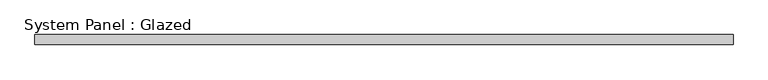
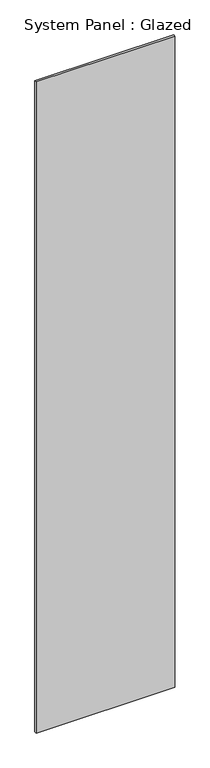
"""IFC4 building model written with IfcOpenShell, lengths in millimetres: plate geometry, System Panel : Glazed."""

from ifc_helpers import new_model, si_unit, origin, origin_with_axes, place, context, project, spatial, polyline, outline, extrude, source, transform, mapped, element, save


def system_panel_glazed_aaff879c(model_context):
    return source(origin(), model_context, "Body", "SweptSolid", [
        extrude(outline(polyline([(920.75, 19.05), (-920.75, 19.05), (-920.75, 44.45), (920.75, 44.45), (920.75, 19.05)])), origin_with_axes(), (0.0, 0.0, 1.0), 9144.0),
    ])


if __name__ == "__main__":
    model = new_model("IFC4")
    model_context = context("Model", 3, world=origin())
    ifc_project = project(units=[si_unit("LENGTHUNIT", "METRE", prefix="MILLI")], contexts=[model_context])
    site = spatial("IfcSite", under=ifc_project)
    building = spatial("IfcBuilding", under=site)
    placement = place(None, origin())
    system_panel_glazed_shape = system_panel_glazed_aaff879c(model_context)
    element("IfcPlate", 1, ObjectType="System Panel : Glazed", at=placement, inside=building, context=model_context, shape_type="MappedRepresentation", body=[
        mapped(system_panel_glazed_shape, transform((0.0, 0.0, 0.0), x_axis=(1.0, 0.0, 0.0), y_axis=(0.0, 1.0, 0.0), z_axis=(0.0, 0.0, 1.0))),
    ])
    save(model, "model.ifc")

# Revit data of these elements
# Type "System Panel : Glazed"
#   Construction Type Id = "GSP4R"
#   Analytic Construction = "1/8 in Pilkington single glazing"
#   Visual Light Transmittance = 0.9
#   Solar Heat Gain Coefficient = 0.86
#   Heat Transfer Coefficient (U) = 1.18115 BTU/(h·ft²·°F)
#   Define Thermal Properties by = 1
# Element 1 (IfcPlate, "System Panel : Glazed")
#   Materials on its faces: "Glass"
# Materials
#   "Glass": class "Glass", colour RGB 0 128 192, transparency 0.75, Description = "Soda Lime Glass", Cost = 0
